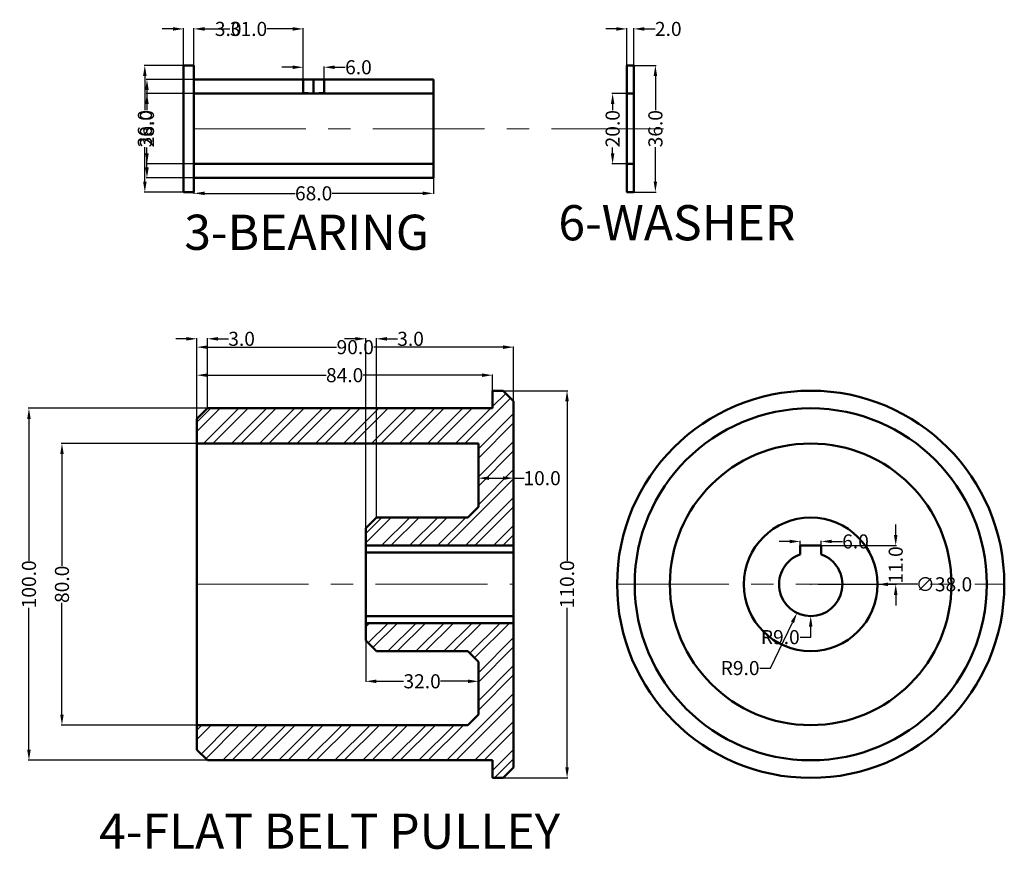
# Model space of a CAD drawing. Units: inches. Extents: x -30 to 602, y 452 to 930.
# Tile 2 of 3: x -2 to 278, y 694 to 930. Entities that reach past the tile are written whole.
import ezdxf

# ---------------------------------------------------------------- set-up
doc = ezdxf.new("R2010")
doc.units = ezdxf.units.IN
doc.header["$MEASUREMENT"] = 0
doc.linetypes.add('CENTER', pattern=[50.8, 31.75, -6.35, 6.35, -6.35])
for name, color, linetype, lineweight in [('M-CNTR', 1, 'CENTER', 18), ('M-DIMS', 2, 'Continuous', 25), ('M-HATC', 8, 'Continuous', 18), ('M-OUTL', 7, 'Continuous', 50), ('M-TEXT', 3, 'Continuous', 25)]:
    doc.layers.add(name, color=color, linetype=linetype, lineweight=lineweight)
doc.styles.get("Standard").update_dxf_attribs({"font": 'arial.ttf'})
doc.dimstyles.get("Standard").update_dxf_attribs({"dimtxt": 4, "dimasz": 3, "dimexe": 0.18, "dimexo": 0.0625, "dimgap": 0.09, "dimtad": 0, "dimtoh": 1, "dimdec": 1, "dimzin": 0, "dimdsep": 46, "dimtxsty": 'Standard', "dimcen": 0.09, "dimadec": 0, "dimazin": 0, "dimtfac": 1, "dimtdec": 1, "dimtofl": 0, "dimtmove": 0, "dimatfit": 3, "dimfxl": 1, "dimtolj": 1, "dimtzin": 0, "dimarcsym": 0})

# ---------------------------------------------------------------- blocks, each defined once
blk = doc.blocks.new('*D1')
at = {"layer": 'Defpoints', "color": 0, "transparency": 16777216}
for p in [(44.5, 917.21), (33.55, 881.21), (44.5, 881.21)]:
    blk.add_point(p, dxfattribs=at)
at = {"layer": 'M-DIMS', "color": 0, "lineweight": -2, "transparency": 16777216}
for p, q in [((44.44, 917.21), (33.37, 917.21)), ((33.55, 914.21), (33.55, 904.48)), ((33.55, 884.21), (33.55, 893.93)), ((44.44, 881.21), (33.37, 881.21))]:
    blk.add_line(p, q, dxfattribs=at)
at = {"layer": 'M-DIMS', "color": 0, "transparency": 16777216}
for points in [[(33.05, 914.21), (34.05, 914.21), (33.55, 917.21)], [(33.05, 884.21), (34.05, 884.21), (33.55, 881.21)]]:
    blk.add_solid(points, dxfattribs=at)
at = {"layer": 'M-DIMS', "color": 0, "transparency": 16777216, "insert": (33.55, 899.21), "char_height": 4, "attachment_point": 5, "rotation": 90}
blk.add_mtext('\\A1;36.0', dxfattribs=at)
blk = doc.blocks.new('*D2')
at = {"layer": 'Defpoints', "color": 0, "transparency": 16777216}
for p in [(115.5, 885.21), (47.5, 883.02), (115.5, 880.85)]:
    blk.add_point(p, dxfattribs=at)
at = {"layer": 'M-DIMS', "color": 0, "lineweight": -2, "transparency": 16777216}
for p, q in [((115.5, 885.15), (115.5, 880.67)), ((47.5, 882.96), (47.5, 880.67)), ((50.5, 880.85), (76.21, 880.85)), ((112.5, 880.85), (86.79, 880.85))]:
    blk.add_line(p, q, dxfattribs=at)
at = {"layer": 'M-DIMS', "color": 0, "transparency": 16777216}
for points in [[(50.5, 881.35), (50.5, 880.35), (47.5, 880.85)], [(112.5, 881.35), (112.5, 880.35), (115.5, 880.85)]]:
    blk.add_solid(points, dxfattribs=at)
at = {"layer": 'M-DIMS', "color": 0, "transparency": 16777216, "insert": (81.5, 880.85), "char_height": 4, "attachment_point": 5}
blk.add_mtext('\\A1;68.0', dxfattribs=at)
blk = doc.blocks.new('*D3')
at = {"layer": 'Defpoints', "color": 0, "transparency": 16777216}
for p in [(84.5, 916.67), (78.5, 912.51), (84.5, 912.29)]:
    blk.add_point(p, dxfattribs=at)
at = {"layer": 'M-DIMS', "color": 0, "lineweight": -2, "transparency": 16777216}
for p, q in [((75.5, 916.67), (72.5, 916.67)), ((78.5, 912.57), (78.5, 916.85)), ((84.5, 912.36), (84.5, 916.85)), ((87.5, 916.67), (90.5, 916.67))]:
    blk.add_line(p, q, dxfattribs=at)
at = {"layer": 'M-DIMS', "color": 0, "transparency": 16777216}
for points in [[(75.5, 917.17), (75.5, 916.17), (78.5, 916.67)], [(87.5, 917.17), (87.5, 916.17), (84.5, 916.67)]]:
    blk.add_solid(points, dxfattribs=at)
at = {"layer": 'M-DIMS', "color": 0, "transparency": 16777216, "insert": (94.23, 916.67), "char_height": 4, "attachment_point": 5}
blk.add_mtext('\\A1;6.0', dxfattribs=at)
blk = doc.blocks.new('*D4')
at = {"layer": 'Defpoints', "color": 0, "transparency": 16777216}
for p in [(171.48, 917.21), (171.48, 881.21), (178.58, 881.21)]:
    blk.add_point(p, dxfattribs=at)
at = {"layer": 'M-DIMS', "color": 0, "lineweight": -2, "transparency": 16777216}
for p, q in [((171.54, 917.21), (178.76, 917.21)), ((178.58, 914.21), (178.58, 904.48)), ((178.58, 884.21), (178.58, 893.93)), ((171.54, 881.21), (178.76, 881.21))]:
    blk.add_line(p, q, dxfattribs=at)
at = {"layer": 'M-DIMS', "color": 0, "transparency": 16777216}
for points in [[(178.08, 914.21), (179.08, 914.21), (178.58, 917.21)], [(178.08, 884.21), (179.08, 884.21), (178.58, 881.21)]]:
    blk.add_solid(points, dxfattribs=at)
at = {"layer": 'M-DIMS', "color": 0, "transparency": 16777216, "insert": (178.58, 899.21), "char_height": 4, "attachment_point": 5, "rotation": 90}
blk.add_mtext('\\A1;36.0', dxfattribs=at)
blk = doc.blocks.new('*D5')
at = {"layer": 'Defpoints', "color": 0, "transparency": 16777216}
for p in [(171.48, 909.21), (166.43, 889.21), (171.48, 889.21)]:
    blk.add_point(p, dxfattribs=at)
at = {"layer": 'M-DIMS', "color": 0, "lineweight": -2, "transparency": 16777216}
for p, q in [((171.41, 909.21), (166.25, 909.21)), ((166.43, 906.21), (166.43, 904.52)), ((166.43, 892.21), (166.43, 893.9)), ((171.41, 889.21), (166.25, 889.21))]:
    blk.add_line(p, q, dxfattribs=at)
at = {"layer": 'M-DIMS', "color": 0, "transparency": 16777216}
for points in [[(165.93, 906.21), (166.93, 906.21), (166.43, 909.21)], [(165.93, 892.21), (166.93, 892.21), (166.43, 889.21)]]:
    blk.add_solid(points, dxfattribs=at)
at = {"layer": 'M-DIMS', "color": 0, "transparency": 16777216, "insert": (166.43, 899.21), "char_height": 4, "attachment_point": 5, "rotation": 90}
blk.add_mtext('\\A1;20.0', dxfattribs=at)
blk = doc.blocks.new('*D6')
at = {"layer": 'Defpoints', "color": 0, "transparency": 16777216}
for p in [(57.03, 819.77), (0.62, 719.77), (57.03, 719.77)]:
    blk.add_point(p, dxfattribs=at)
at = {"layer": 'M-DIMS', "color": 0, "lineweight": -2, "transparency": 16777216}
for p, q in [((56.97, 819.77), (0.44, 819.77)), ((0.62, 816.77), (0.62, 776.41)), ((0.62, 722.77), (0.62, 763.13)), ((56.97, 719.77), (0.44, 719.77))]:
    blk.add_line(p, q, dxfattribs=at)
at = {"layer": 'M-DIMS', "color": 0, "transparency": 16777216}
for points in [[(0.12, 816.77), (1.12, 816.77), (0.62, 819.77)], [(0.12, 722.77), (1.12, 722.77), (0.62, 719.77)]]:
    blk.add_solid(points, dxfattribs=at)
at = {"layer": 'M-DIMS', "color": 0, "transparency": 16777216, "insert": (0.62, 769.77), "char_height": 4, "attachment_point": 5, "rotation": 90}
blk.add_mtext('\\A1;100.0', dxfattribs=at)
blk = doc.blocks.new('*D7')
at = {"layer": 'Defpoints', "color": 0, "transparency": 16777216}
for p in [(48.31, 809.77), (10, 729.77), (48.31, 729.77)]:
    blk.add_point(p, dxfattribs=at)
at = {"layer": 'M-DIMS', "color": 0, "lineweight": -2, "transparency": 16777216}
for p, q in [((48.24, 809.77), (9.82, 809.77)), ((10, 806.77), (10, 775.05)), ((10, 732.77), (10, 764.49)), ((48.24, 729.77), (9.82, 729.77))]:
    blk.add_line(p, q, dxfattribs=at)
at = {"layer": 'M-DIMS', "color": 0, "transparency": 16777216}
for points in [[(9.5, 806.77), (10.5, 806.77), (10, 809.77)], [(9.5, 732.77), (10.5, 732.77), (10, 729.77)]]:
    blk.add_solid(points, dxfattribs=at)
at = {"layer": 'M-DIMS', "color": 0, "transparency": 16777216, "insert": (10, 769.77), "char_height": 4, "attachment_point": 5, "rotation": 90}
blk.add_mtext('\\A1;80.0', dxfattribs=at)
blk = doc.blocks.new('*D8')
at = {"layer": 'Defpoints', "color": 0, "transparency": 16777216}
for p in [(134.54, 824.77), (133.81, 714.77), (153.49, 714.77)]:
    blk.add_point(p, dxfattribs=at)
at = {"layer": 'M-DIMS', "color": 0, "lineweight": -2, "transparency": 16777216}
for p, q in [((134.6, 824.77), (153.67, 824.77)), ((153.49, 821.77), (153.49, 776.41)), ((153.49, 717.77), (153.49, 763.13)), ((133.87, 714.77), (153.67, 714.77))]:
    blk.add_line(p, q, dxfattribs=at)
at = {"layer": 'M-DIMS', "color": 0, "transparency": 16777216}
for points in [[(152.99, 821.77), (153.99, 821.77), (153.49, 824.77)], [(152.99, 717.77), (153.99, 717.77), (153.49, 714.77)]]:
    blk.add_solid(points, dxfattribs=at)
at = {"layer": 'M-DIMS', "color": 0, "transparency": 16777216, "insert": (153.49, 769.77), "char_height": 4, "attachment_point": 5, "rotation": 90}
blk.add_mtext('\\A1;110.0', dxfattribs=at)
blk = doc.blocks.new('*D9')
at = {"layer": 'Defpoints', "color": 0, "transparency": 16777216}
for p in [(96.31, 765.39), (96.31, 742.22), (128.31, 740.27)]:
    blk.add_point(p, dxfattribs=at)
at = {"layer": 'M-DIMS', "color": 0, "lineweight": -2, "transparency": 16777216}
for p, q in [((96.31, 765.33), (96.31, 742.04)), ((99.31, 742.22), (107.03, 742.22)), ((125.31, 742.22), (117.58, 742.22)), ((128.31, 740.33), (128.31, 742.4))]:
    blk.add_line(p, q, dxfattribs=at)
at = {"layer": 'M-DIMS', "color": 0, "transparency": 16777216}
for points in [[(99.31, 742.72), (99.31, 741.72), (96.31, 742.22)], [(125.31, 742.72), (125.31, 741.72), (128.31, 742.22)]]:
    blk.add_solid(points, dxfattribs=at)
at = {"layer": 'M-DIMS', "color": 0, "transparency": 16777216, "insert": (112.31, 742.22), "char_height": 4, "attachment_point": 5}
blk.add_mtext('\\A1;32.0', dxfattribs=at)
blk = doc.blocks.new('*D10')
at = {"layer": 'Defpoints', "color": 0, "transparency": 16777216}
for p in [(128.31, 803.37), (138.31, 803.37), (138.31, 799.93)]:
    blk.add_point(p, dxfattribs=at)
at = {"layer": 'M-DIMS', "color": 0, "lineweight": -2, "transparency": 16777216}
for p, q in [((128.31, 803.31), (128.31, 799.75)), ((138.31, 803.31), (138.31, 799.75)), ((131.31, 799.93), (135.31, 799.93)), ((138.31, 799.93), (141.31, 799.93))]:
    blk.add_line(p, q, dxfattribs=at)
at = {"layer": 'M-DIMS', "color": 0, "transparency": 16777216}
for points in [[(131.31, 800.43), (131.31, 799.43), (128.31, 799.93)], [(135.31, 800.43), (135.31, 799.43), (138.31, 799.93)]]:
    blk.add_solid(points, dxfattribs=at)
at = {"layer": 'M-DIMS', "color": 0, "transparency": 16777216, "insert": (146.4, 799.93), "char_height": 4, "attachment_point": 5}
blk.add_mtext('\\A1;10.0', dxfattribs=at)
blk = doc.blocks.new('*D11')
at = {"layer": 'Defpoints', "color": 0, "transparency": 16777216}
for p in [(48.31, 829.19), (132.31, 822.27), (48.31, 810.87)]:
    blk.add_point(p, dxfattribs=at)
at = {"layer": 'M-DIMS', "color": 0, "lineweight": -2, "transparency": 16777216}
for p, q in [((48.31, 810.93), (48.31, 829.37)), ((51.31, 829.19), (85.02, 829.19)), ((129.31, 829.19), (95.59, 829.19)), ((132.31, 822.33), (132.31, 829.37))]:
    blk.add_line(p, q, dxfattribs=at)
at = {"layer": 'M-DIMS', "color": 0, "transparency": 16777216}
for points in [[(51.31, 829.69), (51.31, 828.69), (48.31, 829.19)], [(129.31, 829.69), (129.31, 828.69), (132.31, 829.19)]]:
    blk.add_solid(points, dxfattribs=at)
at = {"layer": 'M-DIMS', "color": 0, "transparency": 16777216, "insert": (90.31, 829.19), "char_height": 4, "attachment_point": 5}
blk.add_mtext('\\A1;84.0', dxfattribs=at)
blk = doc.blocks.new('*D12')
at = {"layer": 'Defpoints', "color": 0, "transparency": 16777216}
for p in [(48.31, 837.15), (138.31, 818.57), (48.31, 805.56)]:
    blk.add_point(p, dxfattribs=at)
at = {"layer": 'M-DIMS', "color": 0, "lineweight": -2, "transparency": 16777216}
for p, q in [((48.31, 805.63), (48.31, 837.33)), ((51.31, 837.15), (88.03, 837.15)), ((135.31, 837.15), (98.58, 837.15)), ((138.31, 818.63), (138.31, 837.33))]:
    blk.add_line(p, q, dxfattribs=at)
at = {"layer": 'M-DIMS', "color": 0, "transparency": 16777216}
for points in [[(51.31, 837.65), (51.31, 836.65), (48.31, 837.15)], [(135.31, 837.65), (135.31, 836.65), (138.31, 837.15)]]:
    blk.add_solid(points, dxfattribs=at)
at = {"layer": 'M-DIMS', "color": 0, "transparency": 16777216, "insert": (93.31, 837.15), "char_height": 4, "attachment_point": 5}
blk.add_mtext('\\A1;90.0', dxfattribs=at)
blk = doc.blocks.new('*D13')
at = {"layer": 'Defpoints', "color": 0, "transparency": 16777216}
for p in [(225.7, 781.95), (219.7, 779.51), (225.7, 779.51)]:
    blk.add_point(p, dxfattribs=at)
at = {"layer": 'M-DIMS', "color": 0, "lineweight": -2, "transparency": 16777216}
for p, q in [((216.7, 781.95), (213.7, 781.95)), ((219.7, 779.58), (219.7, 782.13)), ((225.7, 779.58), (225.7, 782.13)), ((228.7, 781.95), (231.7, 781.95))]:
    blk.add_line(p, q, dxfattribs=at)
at = {"layer": 'M-DIMS', "color": 0, "transparency": 16777216}
for points in [[(216.7, 782.45), (216.7, 781.45), (219.7, 781.95)], [(228.7, 782.45), (228.7, 781.45), (225.7, 781.95)]]:
    blk.add_solid(points, dxfattribs=at)
at = {"layer": 'M-DIMS', "color": 0, "transparency": 16777216, "insert": (235.43, 781.95), "char_height": 4, "attachment_point": 5}
blk.add_mtext('\\A1;6.0', dxfattribs=at)
blk = doc.blocks.new('*D14')
at = {"layer": 'Defpoints', "color": 0, "transparency": 16777216}
for p in [(224.78, 780.77), (224.78, 769.77), (246.85, 769.77)]:
    blk.add_point(p, dxfattribs=at)
at = {"layer": 'M-DIMS', "color": 0, "lineweight": -2, "transparency": 16777216}
for p, q in [((246.85, 783.77), (246.85, 786.77)), ((224.84, 780.77), (247.03, 780.77)), ((224.84, 769.77), (247.03, 769.77)), ((246.85, 766.77), (246.85, 763.77))]:
    blk.add_line(p, q, dxfattribs=at)
at = {"layer": 'M-DIMS', "color": 0, "transparency": 16777216}
for points in [[(246.35, 783.77), (247.35, 783.77), (246.85, 780.77)], [(246.35, 766.77), (247.35, 766.77), (246.85, 769.77)]]:
    blk.add_solid(points, dxfattribs=at)
at = {"layer": 'M-DIMS', "color": 0, "transparency": 16777216, "insert": (246.85, 775.27), "char_height": 4, "attachment_point": 5, "rotation": 90}
blk.add_mtext('\\A1;11.0', dxfattribs=at)
blk = doc.blocks.new('*D15')
at = {"layer": 'Defpoints', "color": 0, "transparency": 16777216}
for p in [(222.7, 769.77), (218.81, 761.65)]:
    blk.add_point(p, dxfattribs=at)
at = {"layer": 'M-DIMS', "color": 0, "lineweight": -2, "transparency": 16777216}
for p, q in [((222.61, 769.77), (222.79, 769.77)), ((222.7, 769.68), (222.7, 769.86)), ((211.29, 745.98), (217.51, 758.95)), ((208.29, 745.98), (211.29, 745.98))]:
    blk.add_line(p, q, dxfattribs=at)
at = {"layer": 'M-DIMS', "color": 0, "transparency": 16777216}
blk.add_solid([(217.06, 759.17), (217.96, 758.73), (218.81, 761.65)], dxfattribs=at)
at = {"layer": 'M-DIMS', "color": 0, "transparency": 16777216, "insert": (202.65, 745.98), "char_height": 4, "attachment_point": 5}
blk.add_mtext('\\A1;R9.0', dxfattribs=at)
blk = doc.blocks.new('*D51')
at = {"layer": 'Defpoints', "color": 0, "transparency": 16777216}
for p in [(47.5, 913.21), (34.15, 885.21), (47.5, 885.21)]:
    blk.add_point(p, dxfattribs=at)
at = {"layer": 'M-DIMS', "color": 0, "lineweight": -2, "transparency": 16777216}
for p, q in [((47.44, 913.21), (33.97, 913.21)), ((34.15, 910.21), (34.15, 904.52)), ((34.15, 888.21), (34.15, 893.9)), ((47.44, 885.21), (33.97, 885.21))]:
    blk.add_line(p, q, dxfattribs=at)
at = {"layer": 'M-DIMS', "color": 0, "transparency": 16777216}
for points in [[(33.65, 910.21), (34.65, 910.21), (34.15, 913.21)], [(33.65, 888.21), (34.65, 888.21), (34.15, 885.21)]]:
    blk.add_solid(points, dxfattribs=at)
at = {"layer": 'M-DIMS', "color": 0, "transparency": 16777216, "insert": (34.15, 899.21), "char_height": 4, "attachment_point": 5, "rotation": 90}
blk.add_mtext('\\A1;28.0', dxfattribs=at)
blk = doc.blocks.new('*D52')
at = {"layer": 'Defpoints', "color": 0, "transparency": 16777216}
for p in [(47.5, 909.21), (34.15, 889.21), (47.5, 889.21)]:
    blk.add_point(p, dxfattribs=at)
at = {"layer": 'M-DIMS', "color": 0, "lineweight": -2, "transparency": 16777216}
for p, q in [((47.44, 909.21), (33.97, 909.21)), ((34.15, 906.21), (34.15, 904.52)), ((34.15, 892.21), (34.15, 893.9)), ((47.44, 889.21), (33.97, 889.21))]:
    blk.add_line(p, q, dxfattribs=at)
at = {"layer": 'M-DIMS', "color": 0, "transparency": 16777216}
for points in [[(33.65, 906.21), (34.65, 906.21), (34.15, 909.21)], [(33.65, 892.21), (34.65, 892.21), (34.15, 889.21)]]:
    blk.add_solid(points, dxfattribs=at)
at = {"layer": 'M-DIMS', "color": 0, "transparency": 16777216, "insert": (34.15, 899.21), "char_height": 4, "attachment_point": 5, "rotation": 90}
blk.add_mtext('\\A1;20.0', dxfattribs=at)
blk = doc.blocks.new('*D53')
at = {"layer": 'Defpoints', "color": 0, "transparency": 16777216}
for p in [(47.5, 927.56), (44.5, 917.21), (47.5, 917.21)]:
    blk.add_point(p, dxfattribs=at)
at = {"layer": 'M-DIMS', "color": 0, "lineweight": -2, "transparency": 16777216}
for p, q in [((41.5, 927.56), (38.5, 927.56)), ((44.5, 917.27), (44.5, 927.74)), ((47.5, 917.27), (47.5, 927.74)), ((50.5, 927.56), (53.5, 927.56))]:
    blk.add_line(p, q, dxfattribs=at)
at = {"layer": 'M-DIMS', "color": 0, "transparency": 16777216}
for points in [[(41.5, 928.06), (41.5, 927.06), (44.5, 927.56)], [(50.5, 928.06), (50.5, 927.06), (47.5, 927.56)]]:
    blk.add_solid(points, dxfattribs=at)
at = {"layer": 'M-DIMS', "color": 0, "transparency": 16777216, "insert": (57.22, 927.56), "char_height": 4, "attachment_point": 5}
blk.add_mtext('\\A1;3.0', dxfattribs=at)
blk = doc.blocks.new('*D54')
at = {"layer": 'Defpoints', "color": 0, "transparency": 16777216}
for p in [(78.5, 927.56), (47.5, 913.21), (78.5, 913.21)]:
    blk.add_point(p, dxfattribs=at)
at = {"layer": 'M-DIMS', "color": 0, "lineweight": -2, "transparency": 16777216}
for p, q in [((47.5, 913.27), (47.5, 927.74)), ((50.5, 927.56), (57.72, 927.56)), ((75.5, 927.56), (68.28, 927.56)), ((78.5, 913.27), (78.5, 927.74))]:
    blk.add_line(p, q, dxfattribs=at)
at = {"layer": 'M-DIMS', "color": 0, "transparency": 16777216}
for points in [[(50.5, 928.06), (50.5, 927.06), (47.5, 927.56)], [(75.5, 928.06), (75.5, 927.06), (78.5, 927.56)]]:
    blk.add_solid(points, dxfattribs=at)
at = {"layer": 'M-DIMS', "color": 0, "transparency": 16777216, "insert": (63, 927.56), "char_height": 4, "attachment_point": 5}
blk.add_mtext('\\A1;31.0', dxfattribs=at)
blk = doc.blocks.new('*D55')
at = {"layer": 'Defpoints', "color": 0, "transparency": 16777216}
for p in [(172.48, 927.56), (170.48, 917.21), (172.48, 917.21)]:
    blk.add_point(p, dxfattribs=at)
at = {"layer": 'M-DIMS', "color": 0, "lineweight": -2, "transparency": 16777216}
for p, q in [((167.48, 927.56), (164.48, 927.56)), ((170.48, 917.27), (170.48, 927.74)), ((172.48, 917.27), (172.48, 927.74)), ((175.48, 927.56), (178.48, 927.56))]:
    blk.add_line(p, q, dxfattribs=at)
at = {"layer": 'M-DIMS', "color": 0, "transparency": 16777216}
for points in [[(167.48, 928.06), (167.48, 927.06), (170.48, 927.56)], [(175.48, 928.06), (175.48, 927.06), (172.48, 927.56)]]:
    blk.add_solid(points, dxfattribs=at)
at = {"layer": 'M-DIMS', "color": 0, "transparency": 16777216, "insert": (182.24, 927.56), "char_height": 4, "attachment_point": 5}
blk.add_mtext('\\A1;2.0', dxfattribs=at)
blk = doc.blocks.new('*D56')
at = {"layer": 'Defpoints', "color": 0, "transparency": 16777216}
for p in [(51.31, 839.52), (51.31, 819.77), (48.31, 816.77)]:
    blk.add_point(p, dxfattribs=at)
at = {"layer": 'M-DIMS', "color": 0, "lineweight": -2, "transparency": 16777216}
for p, q in [((45.31, 839.52), (42.31, 839.52)), ((48.31, 816.83), (48.31, 839.7)), ((51.31, 819.83), (51.31, 839.7)), ((54.31, 839.52), (57.31, 839.52))]:
    blk.add_line(p, q, dxfattribs=at)
at = {"layer": 'M-DIMS', "color": 0, "transparency": 16777216}
for points in [[(45.31, 840.02), (45.31, 839.02), (48.31, 839.52)], [(54.31, 840.02), (54.31, 839.02), (51.31, 839.52)]]:
    blk.add_solid(points, dxfattribs=at)
at = {"layer": 'M-DIMS', "color": 0, "transparency": 16777216, "insert": (61.03, 839.52), "char_height": 4, "attachment_point": 5}
blk.add_mtext('\\A1;3.0', dxfattribs=at)
blk = doc.blocks.new('*D57')
at = {"layer": 'Defpoints', "color": 0, "transparency": 16777216}
for p in [(99.31, 839.52), (99.31, 788.77), (96.31, 785.77)]:
    blk.add_point(p, dxfattribs=at)
at = {"layer": 'M-DIMS', "color": 0, "lineweight": -2, "transparency": 16777216}
for p, q in [((93.31, 839.52), (90.31, 839.52)), ((96.31, 785.83), (96.31, 839.7)), ((99.31, 788.83), (99.31, 839.7)), ((102.31, 839.52), (105.31, 839.52))]:
    blk.add_line(p, q, dxfattribs=at)
at = {"layer": 'M-DIMS', "color": 0, "transparency": 16777216}
for points in [[(93.31, 840.02), (93.31, 839.02), (96.31, 839.52)], [(102.31, 840.02), (102.31, 839.02), (99.31, 839.52)]]:
    blk.add_solid(points, dxfattribs=at)
at = {"layer": 'M-DIMS', "color": 0, "transparency": 16777216, "insert": (109.03, 839.52), "char_height": 4, "attachment_point": 5}
blk.add_mtext('\\A1;3.0', dxfattribs=at)
blk = doc.blocks.new('*D63')
at = {"layer": 'Defpoints', "color": 0, "transparency": 16777216}
for p in [(203.7, 769.77), (241.7, 769.77)]:
    blk.add_point(p, dxfattribs=at)
at = {"layer": 'M-DIMS', "color": 0, "lineweight": -2, "transparency": 16777216}
for p, q in [((222.61, 769.77), (222.79, 769.77)), ((222.7, 769.68), (222.7, 769.86)), ((253.1, 769.77), (244.7, 769.77))]:
    blk.add_line(p, q, dxfattribs=at)
at = {"layer": 'M-DIMS', "color": 0, "transparency": 16777216}
blk.add_solid([(244.7, 770.27), (244.7, 769.27), (241.7, 769.77)], dxfattribs=at)
at = {"layer": 'M-DIMS', "color": 0, "transparency": 16777216, "insert": (260.55, 769.77), "char_height": 4, "attachment_point": 5}
blk.add_mtext('\\A1;∅38.0', dxfattribs=at)
blk = doc.blocks.new('*D64')
at = {"layer": 'Defpoints', "color": 0, "transparency": 16777216}
for p in [(222.7, 769.77), (222.7, 760.77)]:
    blk.add_point(p, dxfattribs=at)
at = {"layer": 'M-DIMS', "color": 0, "lineweight": -2, "transparency": 16777216}
for p, q in [((222.61, 769.77), (222.79, 769.77)), ((222.7, 769.68), (222.7, 769.86)), ((222.7, 754.77), (222.7, 757.77)), ((219.7, 754.77), (222.7, 754.77))]:
    blk.add_line(p, q, dxfattribs=at)
at = {"layer": 'M-DIMS', "color": 0, "transparency": 16777216}
blk.add_solid([(222.2, 757.77), (223.2, 757.77), (222.7, 760.77)], dxfattribs=at)
at = {"layer": 'M-DIMS', "color": 0, "transparency": 16777216, "insert": (214.06, 754.77), "char_height": 4, "attachment_point": 5}
blk.add_mtext('\\A1;R9.0', dxfattribs=at)

msp = doc.modelspace()

# ---------------------------------------------------------------- hatches: boundary and pattern name
at = {"layer": 'M-HATC'}
h = msp.add_hatch(dxfattribs=at)
h.set_pattern_fill('ANSI32', color=256, scale=15)
h.set_pattern_definition([(45, (0, -28), (-3.977476, 3.977476), []), (45, (2.6517, -28), (-3.977476, 3.977476), [])])
h.paths.add_polyline_path([(132.31, 719.77), (132.31, 714.77), (135.31, 714.77), (138.31, 717.77), (138.31, 758.77), (96.31, 758.77), (96.31, 753.77), (99.31, 750.77), (125.31, 750.77), (128.31, 747.77), (128.31, 732.77), (125.31, 729.77), (48.31, 729.77), (48.31, 722.77), (51.31, 719.77)])
h.paths.add_polyline_path([(128.31, 809.77), (128.31, 791.77), (125.31, 788.77), (99.31, 788.77), (96.31, 785.77), (96.31, 780.77), (138.31, 780.77), (138.31, 821.77), (135.31, 824.77), (132.31, 824.77), (132.31, 819.77), (51.31, 819.77), (48.31, 816.77), (48.31, 809.77)])

# ---------------------------------------------------------------- linework, layer by layer
at = {"layer": 'M-CNTR'}
for p, q in [((47.5, 899.21), (184.49, 899.21)), ((48.31, 769.77), (138.31, 769.77)), ((167.7, 769.77), (277.7, 769.77))]:
    msp.add_line(p, q, dxfattribs=at)
at = {"layer": 'M-OUTL'}
for p, q in [((44.5, 917.21), (47.5, 917.21)), ((44.5, 881.21), (44.5, 917.21)), ((47.5, 917.21), (47.5, 881.21)), ((115.5, 913.21), (47.5, 913.21)), ((78.5, 909.21), (78.5, 913.21)), ((81.5, 909.21), (81.5, 913.21)), ((84.5, 909.21), (84.5, 913.21)), ((115.5, 885.21), (115.5, 913.21)), ((115.5, 909.21), (47.5, 909.21)), ((81.5, 909.21), (78.5, 909.38)), ((81.5, 909.21), (84.5, 909.38)), ((170.48, 909.21), (172.48, 909.21)), ((115.5, 889.21), (47.5, 889.21)), ((170.48, 889.21), (172.48, 889.21)), ((115.5, 885.21), (47.5, 885.21)), ((47.5, 881.21), (44.5, 881.21)), ((132.31, 819.77), (132.31, 824.77)), ((132.31, 824.77), (135.31, 824.77)), ((135.31, 824.77), (138.31, 821.77)), ((51.31, 819.77), (48.31, 816.77)), ((51.31, 819.77), (132.31, 819.77)), ((138.31, 821.77), (138.31, 717.77)), ((48.31, 722.77), (48.31, 816.77)), ((48.31, 809.77), (128.31, 809.77)), ((128.31, 809.77), (128.31, 791.77)), ((125.31, 788.77), (128.31, 791.77)), ((96.31, 785.77), (99.31, 788.77)), ((99.31, 788.77), (125.31, 788.77)), ((96.31, 785.77), (96.31, 753.77)), ((96.31, 780.77), (138.31, 780.77)), ((219.7, 778.26), (219.7, 780.77)), ((219.7, 780.77), (225.7, 780.77)), ((225.7, 778.26), (225.7, 780.77)), ((138.31, 778.77), (96.31, 778.77)), ((138.31, 760.77), (96.31, 760.77)), ((96.31, 758.77), (138.31, 758.77)), ((96.31, 753.77), (99.31, 750.77)), ((99.31, 750.77), (125.31, 750.77)), ((125.31, 750.77), (128.31, 747.77)), ((128.31, 747.77), (128.31, 732.77)), ((125.31, 729.77), (128.31, 732.77)), ((48.31, 729.77), (125.31, 729.77)), ((48.31, 722.77), (51.31, 719.77)), ((132.31, 719.77), (51.31, 719.77)), ((132.31, 714.77), (132.31, 719.77)), ((138.31, 717.77), (135.31, 714.77)), ((135.31, 714.77), (132.31, 714.77))]:
    msp.add_line(p, q, dxfattribs=at)
msp.add_lwpolyline([(170.48, 917.21), (172.48, 917.21), (172.48, 881.21), (170.48, 881.21)], close=True, dxfattribs=at)
for radius in [55, 50, 40, 19]:
    msp.add_circle((222.7, 769.77), radius, dxfattribs=at)
msp.add_arc((222.7, 769.77), 9, 109.4712, 70.5288, dxfattribs=at)

# ---------------------------------------------------------------- texts
at = {"layer": 'M-TEXT'}
for s, p in [('6-WASHER', (151.02, 867.5)), ('3-BEARING', (44.75, 864.79)), ('4-FLAT BELT PULLEY', (20.57, 694.66))]:
    msp.add_text(s, height=10, dxfattribs=at).set_placement(p)

# ---------------------------------------------------------------- dimensions: what is measured, and where the dimension line sits
at = {"layer": 'M-DIMS'}
for base, p1, p2, override, picture, middle in [((47.5, 927.56), (44.5, 917.21), (47.5, 917.21), {"dimdec": 1, "dimlfac": 1, "dimrnd": 0, "dimzin": 0, "dimdsep": 46, "dimlunit": 2}, '*D53', (57.22, 927.56)), ((78.5, 927.56), (47.5, 913.21), (78.5, 913.21), {"dimdec": 1, "dimlfac": 1, "dimrnd": 0, "dimzin": 0, "dimdsep": 46, "dimlunit": 2}, '*D54', (63, 927.56)), ((172.48, 927.56), (170.48, 917.21), (172.48, 917.21), {"dimdec": 1, "dimlfac": 1, "dimrnd": 0, "dimzin": 0, "dimdsep": 46, "dimlunit": 2}, '*D55', (182.24, 927.56)), ((84.5, 916.67), (78.5, 912.51), (84.5, 912.29), {"dimclrd": 0, "dimclre": 0, "dimclrt": 0}, '*D3', (94.23, 916.67)), ((115.5, 880.85), (47.5, 883.02), (115.5, 885.21), {"dimclrd": 0, "dimclre": 0, "dimclrt": 0}, '*D2', (81.5, 880.85)), ((51.31, 839.52), (48.31, 816.77), (51.31, 819.77), {"dimdec": 1, "dimlfac": 1, "dimrnd": 0, "dimzin": 0, "dimdsep": 46, "dimlunit": 2}, '*D56', (61.03, 839.52)), ((99.31, 839.52), (96.31, 785.77), (99.31, 788.77), {"dimdec": 1, "dimlfac": 1, "dimrnd": 0, "dimzin": 0, "dimdsep": 46, "dimlunit": 2}, '*D57', (109.03, 839.52)), ((48.31, 837.15), (138.31, 818.57), (48.31, 805.56), {"dimclrd": 0, "dimclre": 0, "dimclrt": 0}, '*D12', (93.31, 837.15)), ((48.31, 829.19), (132.31, 822.27), (48.31, 810.87), {"dimclrd": 0, "dimclre": 0, "dimclrt": 0}, '*D11', (90.31, 829.19)), ((138.31, 799.93), (128.31, 803.37), (138.31, 803.37), {"dimclrd": 0, "dimclre": 0, "dimclrt": 0}, '*D10', (146.4, 799.93)), ((225.7, 781.95), (219.7, 779.51), (225.7, 779.51), {"dimclrd": 0, "dimclre": 0, "dimclrt": 0}, '*D13', (235.43, 781.95)), ((96.31, 742.22), (128.31, 740.27), (96.31, 765.39), {"dimclrd": 0, "dimclre": 0, "dimclrt": 0}, '*D9', (112.31, 742.22))]:
    dim = msp.add_linear_dim(base=base, p1=p1, p2=p2, dimstyle='Standard', override=override, dxfattribs=at)
    dim.commit()
    dim.dimension.update_dxf_attribs({"geometry": picture, "text_midpoint": middle})
for base, p1, p2, override, picture, middle in [((33.55, 881.21), (44.5, 917.21), (44.5, 881.21), {"dimclrd": 0, "dimclre": 0, "dimclrt": 0}, '*D1', (33.55, 899.21)), ((178.58, 881.21), (171.48, 917.21), (171.48, 881.21), {"dimclrd": 0, "dimclre": 0, "dimclrt": 0}, '*D4', (178.58, 899.21)), ((34.15, 885.21), (47.5, 913.21), (47.5, 885.21), {"dimdec": 1, "dimlfac": 1, "dimrnd": 0, "dimzin": 0, "dimdsep": 46, "dimlunit": 2}, '*D51', (34.15, 899.21)), ((34.15, 889.21), (47.5, 909.21), (47.5, 889.21), {"dimdec": 1, "dimlfac": 1, "dimrnd": 0, "dimzin": 0, "dimdsep": 46, "dimlunit": 2}, '*D52', (34.15, 899.21)), ((166.43, 889.21), (171.48, 909.21), (171.48, 889.21), {"dimclrd": 0, "dimclre": 0, "dimclrt": 0}, '*D5', (166.43, 899.21)), ((153.49, 714.77), (134.54, 824.77), (133.81, 714.77), {"dimclrd": 0, "dimclre": 0, "dimclrt": 0}, '*D8', (153.49, 769.77)), ((0.62, 719.77), (57.03, 819.77), (57.03, 719.77), {"dimclrd": 0, "dimclre": 0, "dimclrt": 0}, '*D6', (0.62, 769.77)), ((10, 729.77), (48.31, 809.77), (48.31, 729.77), {"dimclrd": 0, "dimclre": 0, "dimclrt": 0}, '*D7', (10, 769.77)), ((246.85, 769.77), (224.78, 780.77), (224.78, 769.77), {"dimclrd": 0, "dimclre": 0, "dimclrt": 0}, '*D14', (246.85, 775.27))]:
    dim = msp.add_linear_dim(base=base, p1=p1, p2=p2, angle=90, dimstyle='Standard', override=override, dxfattribs=at)
    dim.commit()
    dim.dimension.update_dxf_attribs({"geometry": picture, "text_midpoint": middle})
dim = msp.add_diameter_dim_2p(p1=(203.7, 769.77), p2=(241.7, 769.77), dimstyle='Standard', override={"dimdec": 1, "dimlfac": 1, "dimrnd": 0, "dimzin": 0, "dimdsep": 46, "dimlunit": 2}, dxfattribs=at)
dim.commit()
dim.dimension.update_dxf_attribs({"geometry": '*D63', "text_midpoint": (253.1, 769.77), "dimtype": 163})
dim = msp.add_radius_dim(center=(222.7, 769.77), mpoint=(218.81, 761.65), dimstyle='Standard', override={"dimclrd": 0, "dimclre": 0, "dimclrt": 0}, dxfattribs=at)
dim.commit()
dim.dimension.update_dxf_attribs({"geometry": '*D15', "text_midpoint": (202.65, 745.98), "dimtype": 164})
dim = msp.add_radius_dim(center=(222.7, 769.77), mpoint=(222.7, 760.77), dimstyle='Standard', override={"dimdec": 1, "dimlfac": 1, "dimrnd": 0, "dimzin": 0, "dimdsep": 46, "dimlunit": 2}, dxfattribs=at)
dim.commit()
dim.dimension.update_dxf_attribs({"geometry": '*D64', "text_midpoint": (214.06, 754.77)})

doc.saveas('drawing.dxf')
